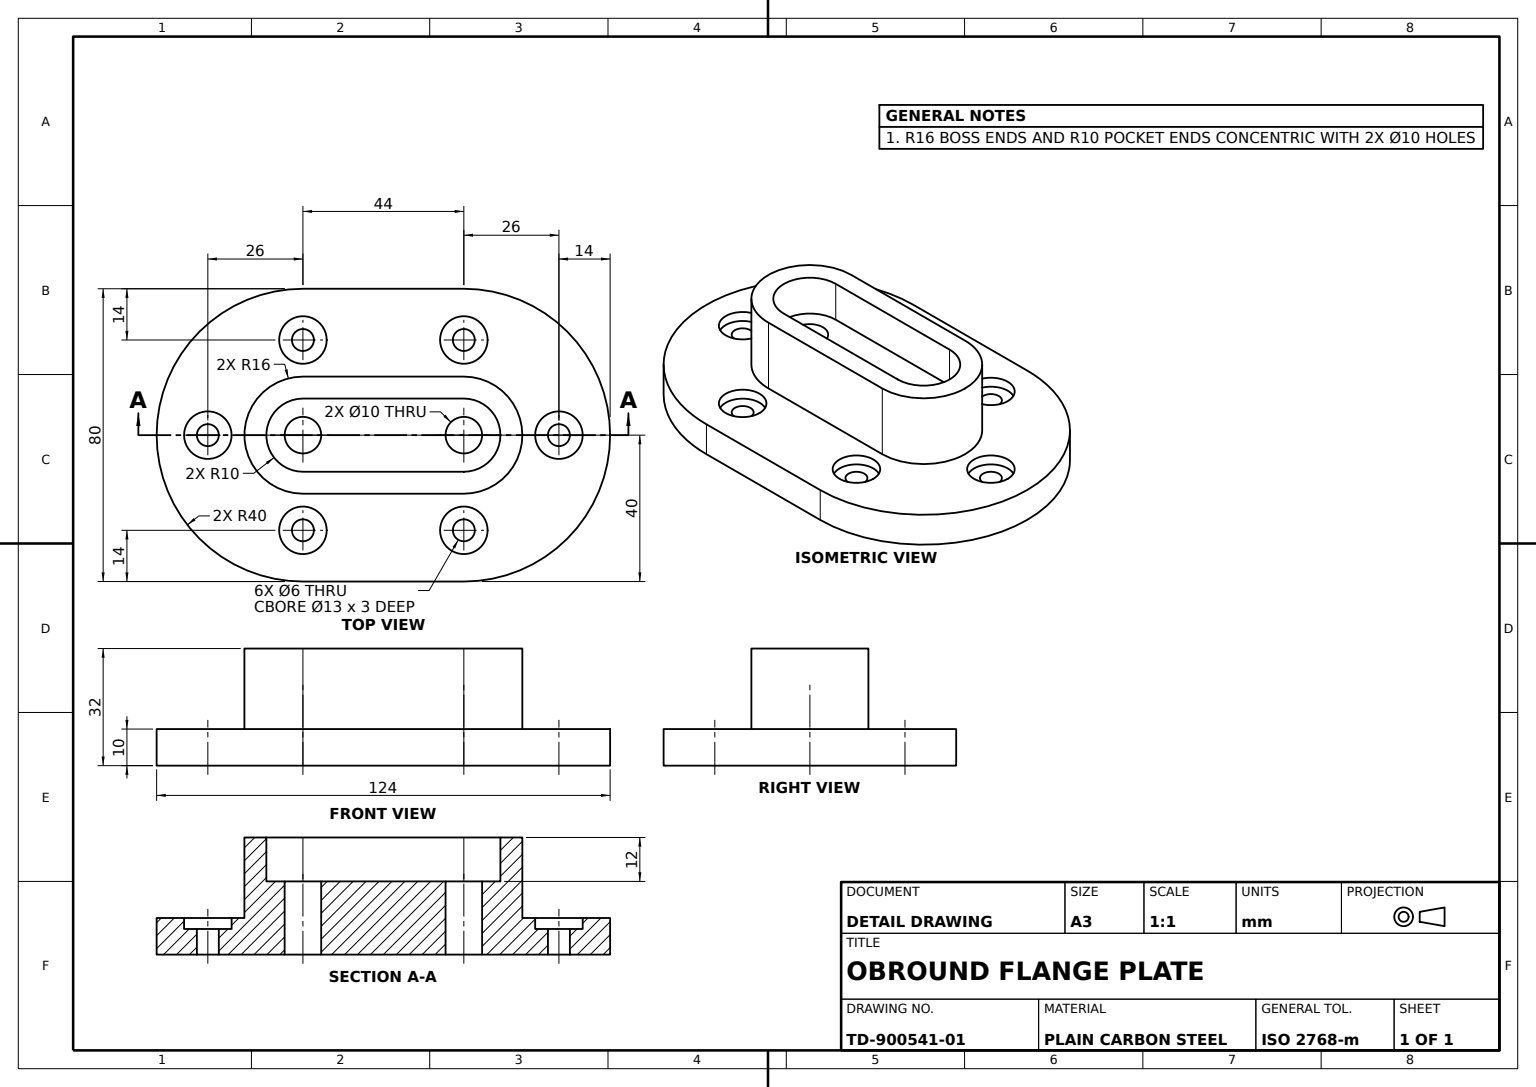
SolidWorks part; units mm, degrees
material "Plain Carbon Steel"
ref_plane "Front Plane" through (0, 0, 0) normal (0, 0, 1) x (1, 0, 0)
ref_plane "Top Plane" through (0, 0, 0) normal (0, 1, 0) x (1, 0, 0)
ref_plane "Right Plane" through (0, 0, 0) normal (1, 0, 0) x (0, 0, -1)
sketch "Base Plate Sketch" plane through (0, 0, 0) normal (0, 1, 0) x (1, 0, 0)
  line L2 (40, 22) -> (40, -22)
  line L3 (-40, 22) -> (-40, -22)
  arc A0 (40, 22) -> (-40, 22) centre (0, 22) ccw
  arc A1 (-40, -22) -> (40, -22) centre (0, -22) ccw
  dimension "D1" = 40
  dimension "D2" = 44
  dimension "D3" = 22
extrude "Base Plate" add sketch "Base Plate Sketch" along normal blind 10
sketch "Slot Boss Sketch" plane through (0, 10, 0) normal (0, 1, 0) x (1, 0, 0)
  line L0 (10, 22) -> (10, -22)
  line L1 (-10, 22) -> (-10, -22)
  line L2 (16, 22) -> (16, -22)
  line L3 (-16, 22) -> (-16, -22)
  line L4 (-40, 22) -> (-40, -22) construction
  arc A1 (16, 22) -> (-16, 22) centre (0, 22) ccw
  arc A2 (-16, -22) -> (16, -22) centre (0, -22) ccw
  arc A3 (10, 22) -> (-10, 22) centre (0, 22) ccw
  arc A4 (-10, -22) -> (10, -22) centre (0, -22) ccw
  dimension "D1" = 16
  dimension "D2" = 10
  dimension "D3" = 40
  dimension "D4" = 44
extrude "Slot Boss" add sketch "Slot Boss Sketch" along normal blind 22
sketch "Secondary Boss Sketch" plane through (0, 10, 0) normal (0, 1, 0) x (1, 0, 0)
  line L2 (-10, 22) -> (-10, -22)
  line L3 (10, -22) -> (10, 22)
  line L4 (-10, 22) -> (-10, -22)
  line L5 (10, -22) -> (10, 22)
  arc A2 (10, 22) -> (-10, 22) centre (0, 22) ccw
  arc A3 (-10, -22) -> (10, -22) centre (0, -22) ccw
  arc A4 (10, 22) -> (-10, 22) centre (0, 22) ccw
  arc A5 (-10, -22) -> (10, -22) centre (0, -22) ccw
  dimension "D1" = 0
extrude "Secondary Boss" add sketch "Secondary Boss Sketch" along normal blind 10
sketch "Slot Cut Sketch" plane through (0, 10, 0) normal (0, 1, 0) x (1, 0, 0)
  circle A0 centre (0, 22) radius 5
  circle A1 centre (0, -22) radius 5
  dimension "D1" = 10
extrude "Slot Through Cut" cut sketch "Slot Cut Sketch" against normal mid plane 69
sketch "Counterbore Sketch" plane through (0, 10, 0) normal (0, 1, 0) x (1, 0, 0)
  line L0 (-40, 22) -> (-40, -22) construction
  circle A0 centre (0, -48) radius 6.5
  circle A1 centre (0, 48) radius 6.5
  circle A2 centre (26, -22) radius 6.5
  circle A3 centre (-26, -22) radius 6.5
  circle A4 centre (26, 22) radius 6.5
  circle A5 centre (-26, 22) radius 6.5
  dimension "D1" = 13
  dimension "D2" = 14
  dimension "D3" = 40
  dimension "D4" = 66
  dimension "D5" = 26
  dimension "D6" = 44
  dimension "D7" = 70
extrude "Counterbores 6x" cut sketch "Counterbore Sketch" against normal blind 3
sketch "Mounting Hole Sketch" plane through (0, 10, 0) normal (0, 1, 0) x (1, 0, 0)
  circle A0 centre (0, -48) radius 3
  circle A1 centre (26, -22) radius 3
  circle A2 centre (26, 22) radius 3
  circle A3 centre (0, 48) radius 3
  circle A4 centre (-26, 22) radius 3
  circle A5 centre (-26, -22) radius 3
  dimension "D1" = 6
extrude "Mounting Holes 6x" cut sketch "Mounting Hole Sketch" against normal blind 88
